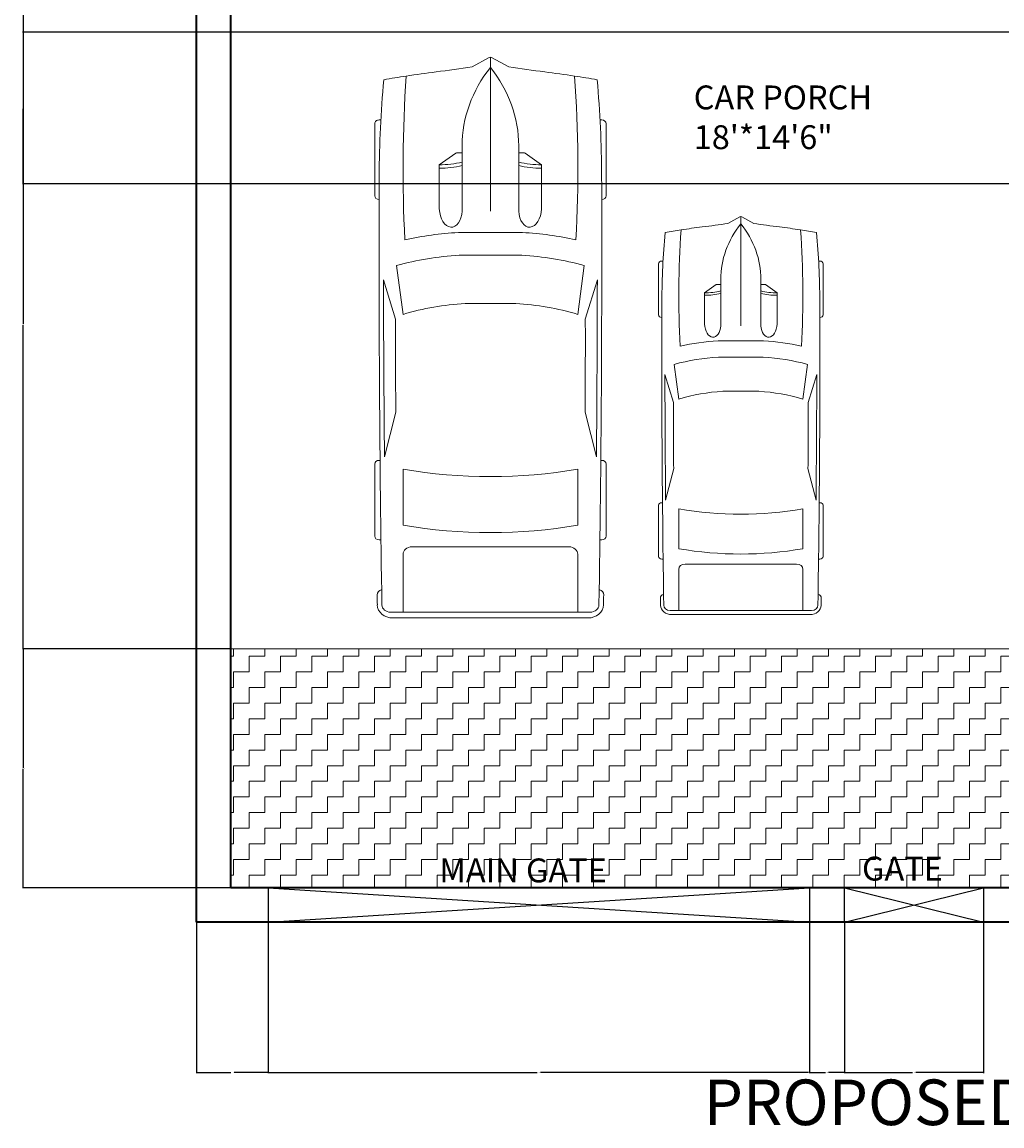
# Model space of a CAD drawing. Units: inches. Extents: x 2284 to 2815, y 1123 to 1948.
# Tile 1 of 6: x 2285 to 2543, y 1123 to 1414. Entities that reach past the tile are written whole.
import ezdxf

# ---------------------------------------------------------------- set-up
doc = ezdxf.new("R2010")
doc.units = ezdxf.units.IN
for name, color, linetype, lineweight in [('A-ANNO-DIMS', 2, 'Continuous', 18), ('A-ANNO-TITL', 30, 'Continuous', 35), ('A-AREA-IDEN', 30, 'Continuous', 18), ('A-WALL-PATT', 140, 'Continuous', 13), ('C-PVMT-PATT', 55, 'Continuous', 13), ('C-SITE-PVMT', 7, 'Continuous', 18), ('C-SITE-VEHC', 8, 'Continuous', 13), ('C-SITE-WALL', 7, 'Continuous', 35), ('L-FENC-GATE', 190, 'Continuous', 25), ('TEXT', 30, 'Continuous', 18)]:
    doc.layers.add(name, color=color, linetype=linetype, lineweight=lineweight)
doc.styles.get("Standard").update_dxf_attribs({"font": 'arial.ttf'})
doc.dimstyles.get("Standard").update_dxf_attribs({"dimtxt": 0.18, "dimasz": 0.18, "dimexe": 0.18, "dimexo": 0.0625, "dimgap": 0.09, "dimtad": 0, "dimtih": 1, "dimtoh": 1, "dimdec": 4, "dimzin": 0, "dimdsep": 46, "dimtxsty": 'Standard', "dimcen": 0.09, "dimadec": 0, "dimazin": 0, "dimtfac": 1, "dimtdec": 4, "dimtofl": 0, "dimtmove": 0, "dimatfit": 3, "dimfxl": 1, "dimtolj": 1, "dimtzin": 0, "dimarcsym": 0})

# ---------------------------------------------------------------- blocks, each defined once
blk = doc.blocks.new('*U8')
for p, q in [((21.1, 37.41), (21.1, 36.83)), ((46.55, 38.89), (22.35, 38.89)), ((47.8, 37.39), (47.8, 37.41)), ((135.45, 37.07), (135.45, 37.41)), ((136.7, 38.89), (160.9, 38.89)), ((162.15, 37.41), (162.15, 36.77)), ((87.99, 31.87), (74.76, 35.92)), ((134.31, 35.6), (119.29, 31.78)), ((186.47, -33.5), (186.47, 33.5)), ((70.03, 31.54), (86.41, 29.35)), ((188.4, -32.76), (188.4, 32.76)), ((138.42, 29.35), (157.25, 29.35)), ((164.52, 26.39), (164.52, -26.39)), ((186.47, 29.35), (167.01, 29.35)), ((32.27, 11.63), (36.13, 17.17)), ((36.13, 17.17), (50.94, 17.17)), ((32.12, 9.51), (32.12, 11.15)), ((29.77, 9.51), (51.68, 9.51)), ((58.92, -10.77), (58.92, 10.77)), ((66.55, -10.53), (66.55, 10.53)), ((82.74, 8.5), (82.74, -8.5)), ((186.47, -10.53), (186.47, 10.53)), ((3.27, 6.13), (0.1, 0.41)), ((0, 0), (51.68, 0)), ((0.1, -0.41), (3.27, -6.13)), ((29.77, -9.51), (51.68, -9.51)), ((32.12, -9.51), (32.12, -11.15)), ((32.27, -11.63), (36.13, -17.17)), ((36.13, -17.17), (50.94, -17.17)), ((86.41, -29.35), (70.03, -31.54)), ((157.25, -29.35), (138.42, -29.35)), ((167.01, -29.35), (186.47, -29.35)), ((87.99, -31.87), (74.76, -35.92)), ((134.31, -35.6), (119.29, -31.78)), ((21.1, -37.41), (21.1, -36.83)), ((135.45, -37.07), (135.45, -37.41)), ((162.15, -37.41), (162.15, -36.77)), ((46.55, -38.89), (22.35, -38.89)), ((47.8, -37.39), (47.8, -37.41)), ((136.7, -38.89), (160.9, -38.89))]:
    blk.add_line(p, q)
for centre, major_axis, ratio, start_param, end_param in [((41.19, -490.86), (0, 528.23), 0.842304, 0.00281, 0.075598), ((22.35, 37.41), (0, -1.48), 0.842304, 3.141593, 4.712389), ((64.48, -10555.62), (0, 10593.03), 0.842304, -0.013397, 0.002797), ((46.55, 37.41), (0, 1.48), 0.842304, -1.570796, 0), ((136.7, 37.41), (0, -1.48), 0.842304, 3.141593, 4.712389), ((160.9, 37.41), (0, 1.48), 0.842304, -1.570796, 0), ((180.63, 35.84), (0, 2.22), 0.842304, -0.013017, 1.249894), ((64.48, -10556.36), (0, 10595.31), 0.842304, -0.013397, -0.013017), ((183.98, 32.76), (0, -5.25), 0.842304, 1.570796, 3.128196), ((266.03, -27.52), (0, 313.31), 0.842304, 1.367076, 1.39176), ((64.48, -10555.62), (0, -10591.55), 0.842304, 3.133765, 3.140441), ((183.98, 33.5), (0, -2.96), 0.842304, 1.570796, 3.128196), ((37.47, -593.96), (0, -623.33), 0.842304, 3.096046, 3.200911), ((135.29, 5.39), (0, 81.77), 0.842304, 1.245306, 1.50788), ((95.79, -3666.35), (0, -3698.24), 0.842304, 3.134049, 3.144098), ((259.18, -27.52), (0, -305.3), 0.842304, 4.528606, 4.561838), ((134.4, 5.39), (0, -89.78), 0.842304, 4.449482, 4.652344), ((149.6, 2.8), (0, -79.58), 0.842304, 4.372215, 4.640744), ((17.08, 0), (0, 147.02), 0.842304, 4.511394, 4.913384), ((35.91, 0), (0, 147.02), 0.842304, 4.511394, 4.913384), ((167.01, 26.39), (0, 2.96), 0.842304, 0, 1.570796), ((-204.49, 52.4), (0, -250.96), 0.842304, 1.385369, 1.434372), ((13.04, 17.01), (0, 27.42), 0.842304, 4.435146, 4.718221), ((14.2, 17.01), (0, 27.42), 0.842304, 4.435146, 4.718221), ((50.79, 13.34), (6.34, -0.36), 0.603834, -1.395552, 1.581315), ((32.75, 11.15), (0, 0.74), 0.842304, 0.879714, 1.570796), ((29.77, -46.66), (0, 56.17), 0.842304, 0, 0.590319), ((0.62, 0), (0, -0.74), 0.842304, 4.131459, 5.293319), ((29.77, 46.66), (0, 56.17), 0.842304, 2.551274, 3.141593), ((-204.49, -52.4), (0, 250.96), 0.842304, -1.434372, -1.385369), ((13.04, -17.01), (0, -27.42), 0.842304, 1.564964, 1.848039), ((14.2, -17.01), (0, -27.42), 0.842304, 1.564964, 1.848039), ((134.4, -5.39), (0, -89.78), 0.842304, -1.510751, -1.307889), ((135.29, -5.39), (0, -81.77), 0.842304, -1.50788, -1.245306), ((149.6, -2.8), (0, -79.58), 0.842304, -1.499151, -1.230623), ((32.75, -11.15), (0, -0.74), 0.842304, 4.712389, 5.403472), ((259.18, 27.52), (0, 305.3), 0.842304, 1.721348, 1.754579), ((266.03, 27.52), (0, 313.31), 0.842304, 1.749832, 1.774517), ((37.47, 593.96), (0, -623.33), 0.842304, -0.059319, 0.045547), ((167.01, -26.39), (0, -2.96), 0.842304, 4.712389, 6.283185), ((95.79, 3666.35), (0, -3698.24), 0.842304, -0.002505, 0.007544), ((183.98, -32.76), (0, -5.25), 0.842304, 0.013397, 1.570796), ((41.19, 490.86), (0, -528.23), 0.842304, -0.075598, -0.00281), ((64.48, 10555.62), (0, 10593.03), 0.842304, 3.138796, 3.15499), ((64.48, 10555.62), (0, -10591.55), 0.842304, 0.001152, 0.007828), ((180.63, -35.84), (0, -2.22), 0.842304, -1.249894, 0.013017), ((183.98, -33.5), (0, 2.96), 0.842304, 3.15499, 4.712389), ((22.35, -37.41), (0, 1.48), 0.842304, 1.570796, 3.141593), ((46.55, -37.41), (0, -1.48), 0.842304, 0, 1.570796), ((136.7, -37.41), (0, -1.48), 0.842304, -1.570796, 0), ((160.9, -37.41), (0, 1.48), 0.842304, 3.141593, 4.712389), ((64.48, 10556.36), (0, 10595.31), 0.842304, 3.15461, 3.15499)]:
    blk.add_ellipse(centre, major_axis=major_axis, ratio=ratio, start_param=start_param, end_param=end_param)
at = {"extrusion": (0, 0, -1)}
blk.add_ellipse((50.79, -13.34), major_axis=(6.34, 0.36), ratio=0.603834, start_param=-1.395552, end_param=1.581315, dxfattribs=at)
blk = doc.blocks.new('*D22')
at = {"layer": 'A-ANNO-DIMS', "color": 0, "lineweight": -2, "transparency": 16777216}
for p, q in [((2339.49, 1248.42), (2284.67, 1248.42)), ((2284.85, 1248.24), (2284.85, 1217.09)), ((2284.85, 1185.58), (2284.85, 1216.73)), ((2339.49, 1185.4), (2284.67, 1185.4))]:
    blk.add_line(p, q, dxfattribs=at)
at = {"layer": 'A-ANNO-DIMS', "color": 0, "transparency": 16777216}
for points in [[(2284.82, 1248.24), (2284.88, 1248.24), (2284.85, 1248.42)], [(2284.82, 1185.58), (2284.88, 1185.58), (2284.85, 1185.4)]]:
    blk.add_solid(points, dxfattribs=at)
at = {"layer": 'Defpoints', "color": 0, "transparency": 16777216}
for p in [(2284.85, 1248.42), (2339.55, 1248.42), (2339.55, 1185.4)]:
    blk.add_point(p, dxfattribs=at)
at = {"layer": 'A-ANNO-DIMS', "color": 0, "transparency": 16777216, "insert": (2284.85, 1216.91), "char_height": 0.18, "attachment_point": 5}
blk.add_mtext('\\A1;63.01', dxfattribs=at)
blk = doc.blocks.new('*D23')
at = {"layer": 'A-ANNO-DIMS', "color": 0, "lineweight": -2, "transparency": 16777216}
for p, q in [((2375.49, 1419.4), (2284.67, 1419.4)), ((2284.85, 1419.22), (2284.85, 1334.09)), ((2284.85, 1248.6), (2284.85, 1333.73)), ((2339.49, 1248.42), (2284.67, 1248.42))]:
    blk.add_line(p, q, dxfattribs=at)
at = {"layer": 'A-ANNO-DIMS', "color": 0, "transparency": 16777216}
for points in [[(2284.82, 1419.22), (2284.88, 1419.22), (2284.85, 1419.4)], [(2284.82, 1248.6), (2284.88, 1248.6), (2284.85, 1248.42)]]:
    blk.add_solid(points, dxfattribs=at)
at = {"layer": 'Defpoints', "color": 0, "transparency": 16777216}
for p in [(2284.85, 1419.4), (2375.55, 1419.4), (2339.55, 1248.42)]:
    blk.add_point(p, dxfattribs=at)
at = {"layer": 'A-ANNO-DIMS', "color": 0, "transparency": 16777216, "insert": (2284.85, 1333.91), "char_height": 0.18, "attachment_point": 5}
blk.add_mtext('\\A1;171', dxfattribs=at)
blk = doc.blocks.new('*D37')
at = {"layer": 'A-ANNO-DIMS', "color": 0, "lineweight": -2, "transparency": 16777216}
for p, q in [((2330.55, 1176.34), (2330.55, 1136.52)), ((2349.43, 1176.34), (2349.43, 1136.52)), ((2330.73, 1136.7), (2339.54, 1136.7)), ((2349.25, 1136.7), (2340.45, 1136.7))]:
    blk.add_line(p, q, dxfattribs=at)
at = {"layer": 'A-ANNO-DIMS', "color": 0, "transparency": 16777216}
for points in [[(2330.73, 1136.73), (2330.73, 1136.67), (2330.55, 1136.7)], [(2349.25, 1136.73), (2349.25, 1136.67), (2349.43, 1136.7)]]:
    blk.add_solid(points, dxfattribs=at)
at = {"layer": 'Defpoints', "color": 0, "transparency": 16777216}
for p in [(2330.55, 1176.4), (2349.43, 1176.4), (2349.43, 1136.7)]:
    blk.add_point(p, dxfattribs=at)
at = {"layer": 'A-ANNO-DIMS', "color": 0, "transparency": 16777216, "insert": (2339.99, 1136.7), "char_height": 0.18, "attachment_point": 5}
blk.add_mtext('\\A1;18.874', dxfattribs=at)
blk = doc.blocks.new('*D38')
at = {"layer": 'A-ANNO-DIMS', "color": 0, "lineweight": -2, "transparency": 16777216}
for p, q in [((2349.43, 1176.34), (2349.43, 1136.52)), ((2492.09, 1176.34), (2492.09, 1136.52)), ((2349.61, 1136.7), (2420.3, 1136.7)), ((2491.91, 1136.7), (2421.21, 1136.7))]:
    blk.add_line(p, q, dxfattribs=at)
at = {"layer": 'A-ANNO-DIMS', "color": 0, "transparency": 16777216}
for points in [[(2349.61, 1136.73), (2349.61, 1136.67), (2349.43, 1136.7)], [(2491.91, 1136.73), (2491.91, 1136.67), (2492.09, 1136.7)]]:
    blk.add_solid(points, dxfattribs=at)
at = {"layer": 'Defpoints', "color": 0, "transparency": 16777216}
for p in [(2349.43, 1176.4), (2492.09, 1176.4), (2492.09, 1136.7)]:
    blk.add_point(p, dxfattribs=at)
at = {"layer": 'A-ANNO-DIMS', "color": 0, "transparency": 16777216, "insert": (2420.76, 1136.7), "char_height": 0.18, "attachment_point": 5}
blk.add_mtext('\\A1;142.66', dxfattribs=at)
blk = doc.blocks.new('*D39')
at = {"layer": 'A-ANNO-DIMS', "color": 0, "lineweight": -2, "transparency": 16777216}
for p, q in [((2492.09, 1176.34), (2492.09, 1136.52)), ((2501.39, 1176.34), (2501.39, 1136.52)), ((2492.27, 1136.7), (2496.35, 1136.7)), ((2501.21, 1136.7), (2497.13, 1136.7))]:
    blk.add_line(p, q, dxfattribs=at)
at = {"layer": 'A-ANNO-DIMS', "color": 0, "transparency": 16777216}
for points in [[(2492.27, 1136.73), (2492.27, 1136.67), (2492.09, 1136.7)], [(2501.21, 1136.73), (2501.21, 1136.67), (2501.39, 1136.7)]]:
    blk.add_solid(points, dxfattribs=at)
at = {"layer": 'Defpoints', "color": 0, "transparency": 16777216}
for p in [(2492.09, 1176.4), (2501.39, 1176.4), (2501.39, 1136.7)]:
    blk.add_point(p, dxfattribs=at)
at = {"layer": 'A-ANNO-DIMS', "color": 0, "transparency": 16777216, "insert": (2496.74, 1136.7), "char_height": 0.18, "attachment_point": 5}
blk.add_mtext('\\A1;9.296', dxfattribs=at)
blk = doc.blocks.new('*D40')
at = {"layer": 'A-ANNO-DIMS', "color": 0, "lineweight": -2, "transparency": 16777216}
for p, q in [((2501.39, 1176.34), (2501.39, 1136.52)), ((2538.03, 1176.34), (2538.03, 1136.52)), ((2501.57, 1136.7), (2519.24, 1136.7)), ((2537.85, 1136.7), (2520.17, 1136.7))]:
    blk.add_line(p, q, dxfattribs=at)
at = {"layer": 'A-ANNO-DIMS', "color": 0, "transparency": 16777216}
for points in [[(2501.57, 1136.73), (2501.57, 1136.67), (2501.39, 1136.7)], [(2537.85, 1136.73), (2537.85, 1136.67), (2538.03, 1136.7)]]:
    blk.add_solid(points, dxfattribs=at)
at = {"layer": 'Defpoints', "color": 0, "transparency": 16777216}
for p in [(2501.39, 1176.4), (2538.03, 1176.4), (2538.03, 1136.7)]:
    blk.add_point(p, dxfattribs=at)
at = {"layer": 'A-ANNO-DIMS', "color": 0, "transparency": 16777216, "insert": (2519.71, 1136.7), "char_height": 0.18, "attachment_point": 5}
blk.add_mtext('\\A1;36.645', dxfattribs=at)
blk = doc.blocks.new('*D47')
at = {"layer": 'A-ANNO-DIMS', "color": 0, "lineweight": -2, "transparency": 16777216}
for p, q in [((2555.49, 1410.98), (2284.67, 1410.98)), ((2284.85, 1410.8), (2284.85, 1391.17)), ((2284.85, 1371.16), (2284.85, 1390.8)), ((2555.49, 1370.98), (2284.67, 1370.98))]:
    blk.add_line(p, q, dxfattribs=at)
at = {"layer": 'A-ANNO-DIMS', "color": 0, "transparency": 16777216}
for points in [[(2284.82, 1410.8), (2284.88, 1410.8), (2284.85, 1410.98)], [(2284.82, 1371.16), (2284.88, 1371.16), (2284.85, 1370.98)]]:
    blk.add_solid(points, dxfattribs=at)
at = {"layer": 'Defpoints', "color": 0, "transparency": 16777216}
for p in [(2284.85, 1410.98), (2555.55, 1410.98), (2555.55, 1370.98)]:
    blk.add_point(p, dxfattribs=at)
at = {"layer": 'A-ANNO-DIMS', "color": 0, "transparency": 16777216, "insert": (2284.85, 1390.98), "char_height": 0.18, "attachment_point": 5}
blk.add_mtext('\\A1;40', dxfattribs=at)

msp = doc.modelspace()

# ---------------------------------------------------------------- hatches: boundary and pattern name
at = {"layer": 'A-WALL-PATT'}
h = msp.add_hatch(dxfattribs=at)
h.set_pattern_fill('AR-SAND', color=256, scale=8.5)
h.paths.add_polyline_path([(2339.554, 1899.404), (2375.554, 1899.404), (2765.554, 1899.404), (2765.554, 1185.404), (2549.3222, 1185.404), (2549.3222, 1176.404), (2774.554, 1176.404), (2774.554, 1908.404), (2330.554, 1908.404), (2330.554, 1176.404), (2349.4276, 1176.404), (2349.4276, 1185.404), (2339.554, 1185.404)])
h.paths.add_polyline_path([(2710.054, 1899.404), (2701.054, 1899.404), (2701.054, 1889.8374), (2710.054, 1889.8374)], flags=17)
h = msp.add_hatch(dxfattribs=at)
h.set_pattern_fill('AR-SAND', color=256, scale=8.5)
h.paths.add_polyline_path([(2549.554, 1863.404), (2375.554, 1863.404), (2375.554, 1840.6021), (2384.554, 1840.6021), (2384.554, 1854.404), (2480.554, 1854.404), (2549.554, 1854.404)])
h.paths.add_polyline_path([(2384.554, 1795.904), (2384.554, 1809.1528), (2375.554, 1809.1528), (2375.554, 1758.7416), (2384.554, 1758.7416)])
h.paths.add_polyline_path([(2549.554, 1836.404), (2549.554, 1854.404), (2540.554, 1854.404), (2540.554, 1800.404), (2485.054, 1800.404), (2485.054, 1802.7347), (2480.554, 1802.7347), (2480.554, 1800.404), (2384.554, 1800.404), (2384.554, 1795.904), (2485.054, 1795.904), (2540.554, 1795.904), (2540.554, 1678.5102), (2543.2164, 1676.3784), (2547.9, 1672.6283), (2549.554, 1677.404), (2549.554, 1795.904)])
h.paths.add_polyline_path([(2452.31, 1803.9815), (2480.7795, 1803.9815), (2480.7795, 1802.7347), (2452.2828, 1802.7347), (2452.2828, 1803.9815), (2452.31, 1803.9815, -0.39915744), (2480.554, 1831.2306), (2480.554, 1854.404), (2540.554, 1854.404), (2485.054, 1837.4988), (2485.054, 1831.2315), (2480.7795, 1831.2315, 0.40145271)], flags=17)
h.paths.add_polyline_path([(2583.189, 1845.404), (2549.554, 1845.404), (2549.554, 1836.404), (2583.189, 1836.404)])
h.paths.add_polyline_path([(2710.054, 1858.3882), (2701.054, 1858.3882), (2701.054, 1845.404), (2671.4007, 1845.404), (2671.4007, 1836.404), (2710.054, 1836.404)])
h.paths.add_polyline_path([(2710.054, 1836.404), (2705.554, 1836.404), (2705.554, 1774.904), (2710.054, 1774.904), (2710.054, 1779.404)])
h.paths.add_polyline_path([(2765.554, 1779.404), (2737.9116, 1779.404, -0.00645116), (2737.9201, 1778.7436), (2737.9201, 1774.904), (2765.554, 1774.904)])
h.paths.add_polyline_path([(2712.3231, 1778.7436), (2712.3231, 1779.404), (2710.054, 1779.404), (2710.054, 1774.904), (2712.3231, 1774.904)])
h.paths.add_polyline_path([(2710.054, 1774.904), (2705.554, 1774.904), (2705.554, 1769.4647), (2710.054, 1769.4647)])
h.paths.add_polyline_path([(2710.054, 1702.7233), (2705.554, 1702.7233), (2705.554, 1686.404), (2592.0733, 1686.404, -0.01876983), (2592.186, 1683.404), (2592.186, 1677.404), (2705.554, 1677.404), (2765.554, 1677.404), (2765.554, 1686.404), (2710.054, 1686.404)])
h.paths.add_polyline_path([(2384.554, 1641.404), (2375.554, 1641.404), (2375.554, 1637.3708), (2381.554, 1637.3708), (2384.554, 1637.3708)])
h.paths.add_polyline_path([(2384.554, 1678.0573), (2375.554, 1678.0573), (2375.554, 1641.404), (2384.554, 1641.404), (2522.8991, 1641.404), (2518.2155, 1645.1541, -0.00736412), (2517.3067, 1645.904), (2384.554, 1645.904)])
h.paths.add_polyline_path([(2384.554, 1597.4834, -0.01876983), (2381.554, 1597.3708), (2375.554, 1597.3708), (2375.554, 1591.564), (2384.554, 1591.564)])
h.paths.add_polyline_path([(2384.554, 1533.404), (2384.554, 1538.4896), (2375.554, 1538.4896), (2375.554, 1524.404), (2384.554, 1524.404)])
h.paths.add_polyline_path([(2506.054, 1533.404), (2506.054, 1598.7748), (2500.054, 1598.7748, -0.01876983), (2497.054, 1598.8874), (2497.054, 1533.404), (2384.554, 1533.404), (2384.554, 1524.404), (2497.054, 1524.404), (2506.054, 1524.404)])
h.paths.add_polyline_path([(2473.054, 1446.985), (2468.9674, 1446.985, -0.00379375), (2468.554, 1446.9881), (2468.554, 1428.404), (2473.054, 1428.404)])
h.paths.add_polyline_path([(2384.554, 1524.404), (2375.554, 1524.404), (2375.554, 1468.4232), (2384.554, 1468.4232)])
h.paths.add_polyline_path([(2473.054, 1480.904), (2384.554, 1480.904), (2384.554, 1476.404), (2468.554, 1476.404), (2468.554, 1474.2289), (2468.9674, 1474.2289), (2473.054, 1474.2289)])
h.paths.add_polyline_path([(2555.554, 1428.404), (2546.554, 1428.404), (2539.1317, 1428.404), (2539.1317, 1422.885), (2539.1317, 1419.404), (2546.554, 1419.404), (2555.554, 1419.404)])
h.paths.add_polyline_path([(2564.554, 1368.404), (2564.554, 1370.9838), (2561.554, 1370.9838), (2555.554, 1370.9838), (2555.554, 1359.404), (2564.554, 1359.404)])
h.paths.add_polyline_path([(2623.1768, 1368.404), (2564.554, 1368.404), (2564.554, 1359.404), (2623.1768, 1359.404)])
h.paths.add_polyline_path([(2492.7181, 1422.885), (2492.7181, 1428.404), (2384.554, 1428.404), (2384.554, 1440.6426), (2375.554, 1440.6426), (2375.554, 1419.404), (2492.7181, 1419.404)])
h.paths.add_polyline_path([(2765.554, 1368.404), (2710.406, 1368.404), (2710.406, 1359.404), (2765.554, 1359.404)])
h.paths.add_polyline_path([(2765.554, 1533.404), (2732.876, 1533.404), (2732.876, 1524.404), (2765.554, 1524.404)])
h.paths.add_polyline_path([(2624.1792, 1533.404), (2599.5288, 1533.404), (2590.3672, 1524.404), (2564.554, 1499.046), (2555.554, 1490.2048), (2555.554, 1410.9838), (2561.554, 1410.9838, -0.01876983), (2564.554, 1410.8712), (2564.554, 1486.4298), (2603.2099, 1524.404), (2624.1792, 1524.404)])
h.paths.add_polyline_path([(2555.554, 1490.2048), (2556.4043, 1491.0401), (2549.047, 1496.8538), (2545.7227, 1492.1958), (2543.8126, 1489.5193), (2555.554, 1480.2413)])
h.paths.add_polyline_path([(2514.6892, 1524.0031), (2506.054, 1530.8266), (2506.054, 1524.404), (2499.6656, 1524.404), (2500.474, 1523.7652), (2509.4548, 1516.6686), (2511.3649, 1519.3451)])
h.paths.add_polyline_path([(2365.9834, 1447.3726), (2374.9891, 1447.3726), (2374.9891, 1460.3342), (2365.9834, 1460.3342)], flags=9)
h.paths.add_polyline_path([(2366.9945, 1818.7713), (2376.0002, 1818.7713), (2376.0002, 1831.7328), (2366.9945, 1831.7328)], flags=9)
h.paths.add_polyline_path([(2363.2989, 1558.2059), (2374.7373, 1558.2059), (2374.7373, 1571.1674), (2363.2989, 1571.1674)], flags=9)
h.paths.add_polyline_path([(2364.8137, 1707.1012), (2376.2521, 1707.1012), (2376.2521, 1720.0627), (2364.8137, 1720.0627)], flags=9)
h.paths.add_polyline_path([(2460.3189, 1455.9932), (2469.8094, 1455.9932), (2469.8094, 1468.9547), (2460.3189, 1468.9547)], flags=9)
h.paths.add_polyline_path([(2558.6325, 1386.2225), (2568.1231, 1386.2225), (2568.1231, 1399.184), (2558.6325, 1399.184)], flags=9)
h.paths.add_polyline_path([(2378.5629, 1611.6816), (2388.0534, 1611.6816), (2388.0534, 1624.6431), (2378.5629, 1624.6431)], flags=9)
h.paths.add_polyline_path([(2490.2277, 1613.2326), (2499.7182, 1613.2326), (2499.7182, 1626.1941), (2490.2277, 1626.1941)], flags=9)
h.paths.add_polyline_path([(2522.9652, 1656.7942), (2532.4557, 1656.7942), (2532.4557, 1669.7557), (2522.9652, 1669.7557)], flags=9)
h.paths.add_polyline_path([(2567.5462, 1677.3031), (2577.0367, 1677.3031), (2577.0367, 1690.2646), (2567.5462, 1690.2646)], flags=9)
h.paths.add_polyline_path([(2363.196, 1676.9136), (2363.196, 1756.4461), (2350.2345, 1756.4461), (2350.2345, 1676.9136)], flags=9)
h.paths.add_polyline_path([(2515.5569, 1505.5998), (2535.7182, 1488.4964), (2539.8301, 1493.3434), (2519.6687, 1510.4468)], flags=9)
h.paths.add_polyline_path([(2503.6006, 1414.6146), (2530.0393, 1414.6146), (2530.0393, 1420.9707), (2503.6006, 1420.9707)], flags=9)
h.paths.add_polyline_path([(2391.2946, 1877.326), (2470.827, 1877.326), (2470.827, 1890.2876), (2391.2946, 1890.2876)], flags=9)
h.paths.add_polyline_path([(2580.3233, 1794.4386), (2629.1831, 1794.4386), (2629.1831, 1817.9089), (2580.3233, 1817.9089)], flags=9)
h.paths.add_polyline_path([(2585.6043, 1595.2228), (2648.3653, 1595.2228), (2648.3653, 1618.6931), (2585.6043, 1618.6931)], flags=9)
h.paths.add_polyline_path([(2591.9981, 1445.0189), (2637.889, 1445.0189), (2637.889, 1468.4892), (2591.9981, 1468.4892)], flags=9)
h.paths.add_polyline_path([(2459.0727, 1376.5795), (2515.4624, 1376.5795), (2515.4624, 1400.0498), (2459.0727, 1400.0498)], flags=9)
h.paths.add_polyline_path([(2481.8769, 1451.6363), (2543.2049, 1451.6363), (2543.2049, 1475.1066), (2481.8769, 1475.1066)], flags=9)
h.paths.add_polyline_path([(2470.0329, 1495.943), (2485.3842, 1495.943), (2485.3842, 1508.9045), (2470.0329, 1508.9045)], flags=9)
h.paths.add_polyline_path([(2419.5143, 1438.0898), (2446.0938, 1438.0898), (2446.0938, 1461.5344), (2419.5143, 1461.5344)], flags=9)
h.paths.add_polyline_path([(2425.6893, 1570.7133), (2467.4012, 1570.7133), (2467.4012, 1594.1836), (2425.6893, 1594.1836)], flags=25)
h.paths.add_polyline_path([(2428.101, 1758.2973), (2476.9609, 1758.2973), (2476.9609, 1781.7676), (2428.101, 1781.7676)], flags=25)
at = {"layer": 'C-PVMT-PATT'}
h = msp.add_hatch(dxfattribs=at)
h.set_pattern_fill('ZIGZAG', color=256, scale=1.3)
h.set_pattern_definition([(0, (0, 0), (4.1275, 4.1275), [4.1275, -4.1275]), (90, (4.1275, 0), (-4.1275, 4.1275), [4.1275, -4.1275])])
h.paths.add_polyline_path([(2564.554, 1248.417), (2339.554, 1248.417), (2339.554, 1185.404), (2564.554, 1185.404)])

# ---------------------------------------------------------------- linework, layer by layer
at = {"layer": 'C-SITE-PVMT'}
msp.add_line((2339.554, 1248.417), (2564.554, 1248.417), dxfattribs=at)
at = {"layer": 'C-SITE-WALL'}
for p, q in [((2330.554, 1176.404), (2330.554, 1908.404)), ((2339.554, 1185.404), (2339.554, 1899.404)), ((2765.554, 1185.404), (2339.554, 1185.404)), ((2774.554, 1176.404), (2330.554, 1176.404))]:
    msp.add_line(p, q, dxfattribs=at)
at = {"layer": 'L-FENC-GATE'}
for p, q in [((2349.4276, 1185.404), (2349.4276, 1176.404)), ((2349.4276, 1176.404), (2492.0911, 1185.404)), ((2349.4276, 1185.404), (2492.0911, 1176.404)), ((2501.3868, 1176.404), (2538.0313, 1185.404)), ((2501.3868, 1185.404), (2538.0313, 1176.404)), ((2538.0313, 1185.404), (2538.0313, 1176.404))]:
    msp.add_line(p, q, dxfattribs=at)
msp.add_lwpolyline([(2501.3868, 1185.404), (2492.0911, 1185.404), (2492.0911, 1176.404), (2501.3868, 1176.404)], close=True, dxfattribs=at)

# ---------------------------------------------------------------- block references
at = {"layer": 'C-SITE-VEHC', "rotation": 270}
for p, xscale, yscale, zscale in [((2408.0166, 1404.3865), 0.7846265055318319, 0.7846265055318319, 0.7846265055318319), ((2474.0292, 1362.3934), 0.557019042196941, 0.557019042196941, 0.557019042196941)]:
    msp.add_blockref('*U8', p, dxfattribs=dict(at, xscale=xscale, yscale=yscale, zscale=zscale))

# ---------------------------------------------------------------- texts
at = {"layer": 'A-ANNO-TITL', "insert": (2464.2261, 1134.8759), "char_height": 12.014871, "attachment_point": 1}
msp.add_mtext_dynamic_manual_height_columns('PROPOSED GROUND FLOOR', width=350.083049, gutter_width=60.0744, heights=[0], dxfattribs=at)
at = {"layer": 'A-AREA-IDEN', "insert": (2461.602, 1396.9242), "char_height": 6.28983, "attachment_point": 1}
msp.add_mtext_dynamic_manual_height_columns('CAR PORCH\\P18\'*14\'6"', width=114.078767, gutter_width=31.4491, heights=[0], dxfattribs=at)
at = {"layer": 'TEXT', "char_height": 6.28983, "attachment_point": 1}
for s, insert in [('MAIN GATE', (2394.5719, 1193.148)), ('GATE', (2505.9772, 1193.62))]:
    msp.add_mtext_dynamic_manual_height_columns(s, width=114.078767, gutter_width=31.4491, heights=[0], dxfattribs=dict(at, insert=insert))

# ---------------------------------------------------------------- dimensions: what is measured, and where the dimension line sits
at = {"layer": 'A-ANNO-DIMS'}
for base, p1, p2, override, picture, middle in [((2284.854, 1419.404), (2339.554, 1248.417), (2375.554, 1419.404), {"dimdec": 0, "dimlfac": 1, "dimrnd": 0, "dimzin": 0, "dimdsep": 46, "dimlunit": 2}, '*D23', (2284.854, 1333.9105)), ((2284.854, 1410.9838), (2555.554, 1370.9838), (2555.554, 1410.9838), {"dimdec": 0, "dimlfac": 1, "dimrnd": 0, "dimzin": 0, "dimdsep": 46, "dimlunit": 2}, '*D47', (2284.854, 1390.9838)), ((2284.854, 1248.417), (2339.554, 1185.404), (2339.554, 1248.417), {"dimdec": 2, "dimlfac": 1, "dimrnd": 0, "dimzin": 0, "dimdsep": 46, "dimlunit": 2}, '*D22', (2284.854, 1216.9105))]:
    dim = msp.add_linear_dim(base=base, p1=p1, p2=p2, angle=90, dimstyle='Standard', override=override, dxfattribs=at)
    dim.commit()
    dim.dimension.update_dxf_attribs({"geometry": picture, "text_midpoint": middle})
for base, p1, p2, override, picture, middle in [((2349.4276, 1136.704), (2330.554, 1176.404), (2349.4276, 1176.404), {"dimdec": 3, "dimlfac": 1, "dimrnd": 0, "dimzin": 0, "dimdsep": 46, "dimlunit": 2}, '*D37', (2339.9908, 1136.704)), ((2492.0911, 1136.704), (2349.4276, 1176.404), (2492.0911, 1176.404), {"dimdec": 2, "dimlfac": 1, "dimrnd": 0, "dimzin": 0, "dimdsep": 46, "dimlunit": 2}, '*D38', (2420.7594, 1136.704)), ((2501.3868, 1136.704), (2492.0911, 1176.404), (2501.3868, 1176.404), {"dimdec": 3, "dimlfac": 1, "dimrnd": 0, "dimzin": 0, "dimdsep": 46, "dimlunit": 2}, '*D39', (2496.7389, 1136.704)), ((2538.03132, 1136.70399), (2501.38676, 1176.40399), (2538.03132, 1176.40399), {"dimdec": 3, "dimlfac": 1, "dimrnd": 0, "dimzin": 0, "dimdsep": 46, "dimlunit": 2}, '*D40', (2519.70904, 1136.70399))]:
    dim = msp.add_linear_dim(base=base, p1=p1, p2=p2, dimstyle='Standard', override=override, dxfattribs=at)
    dim.commit()
    dim.dimension.update_dxf_attribs({"geometry": picture, "text_midpoint": middle})

doc.saveas('drawing.dxf')
